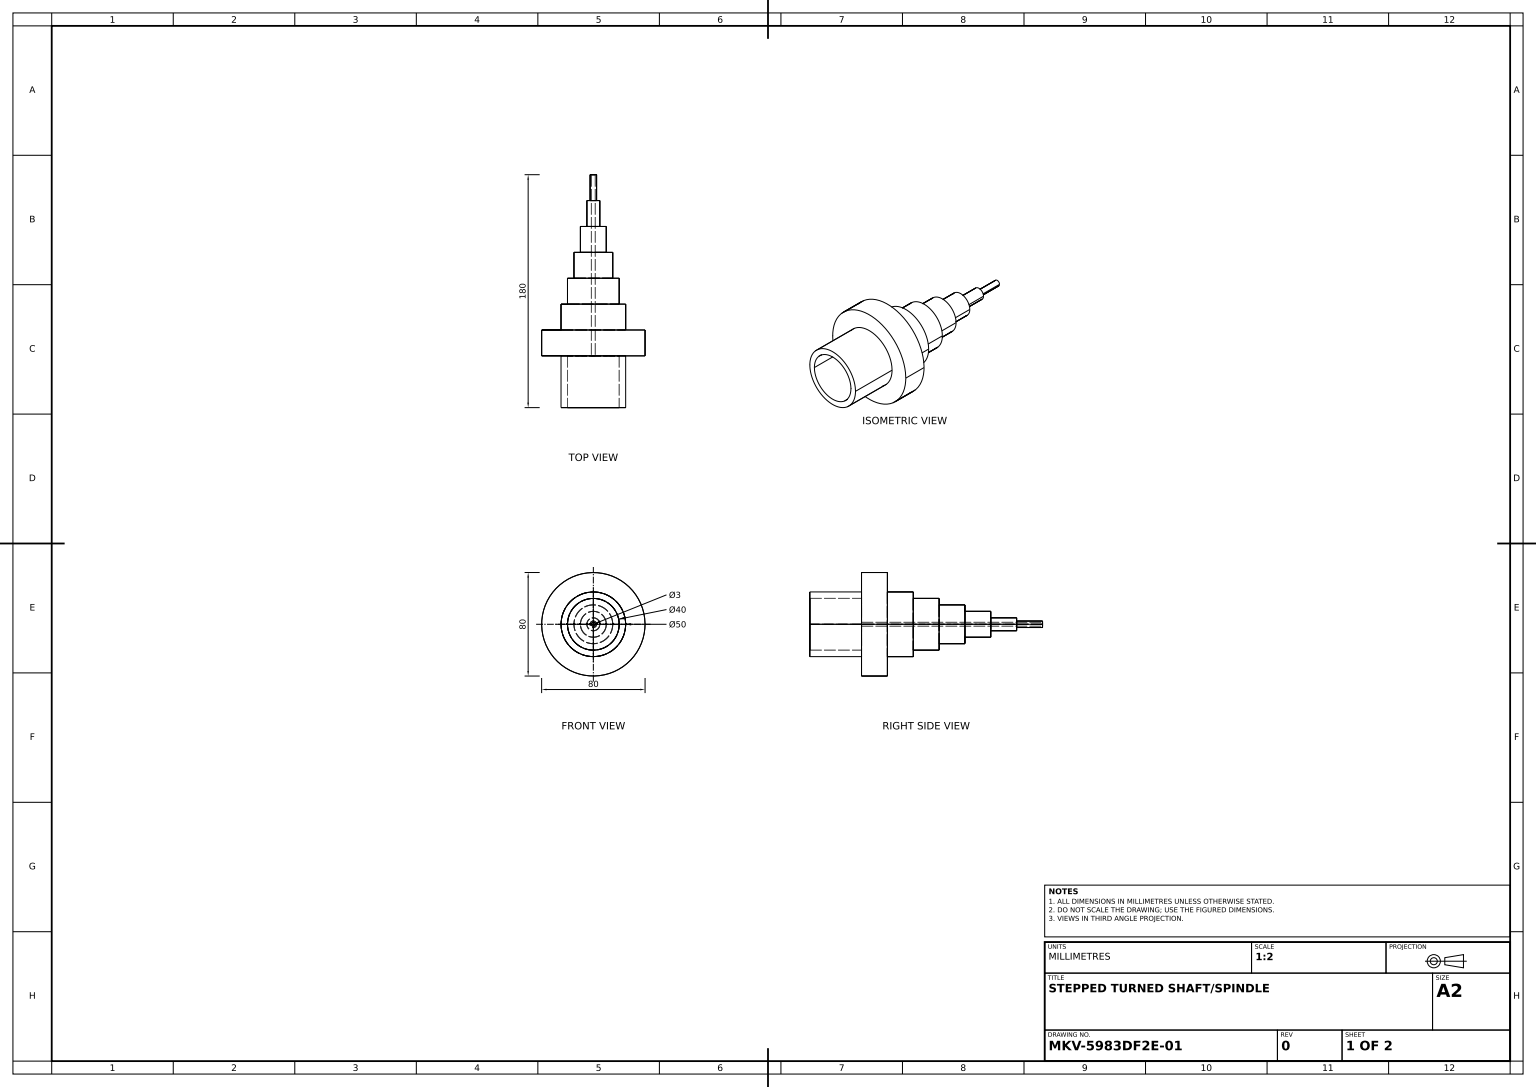
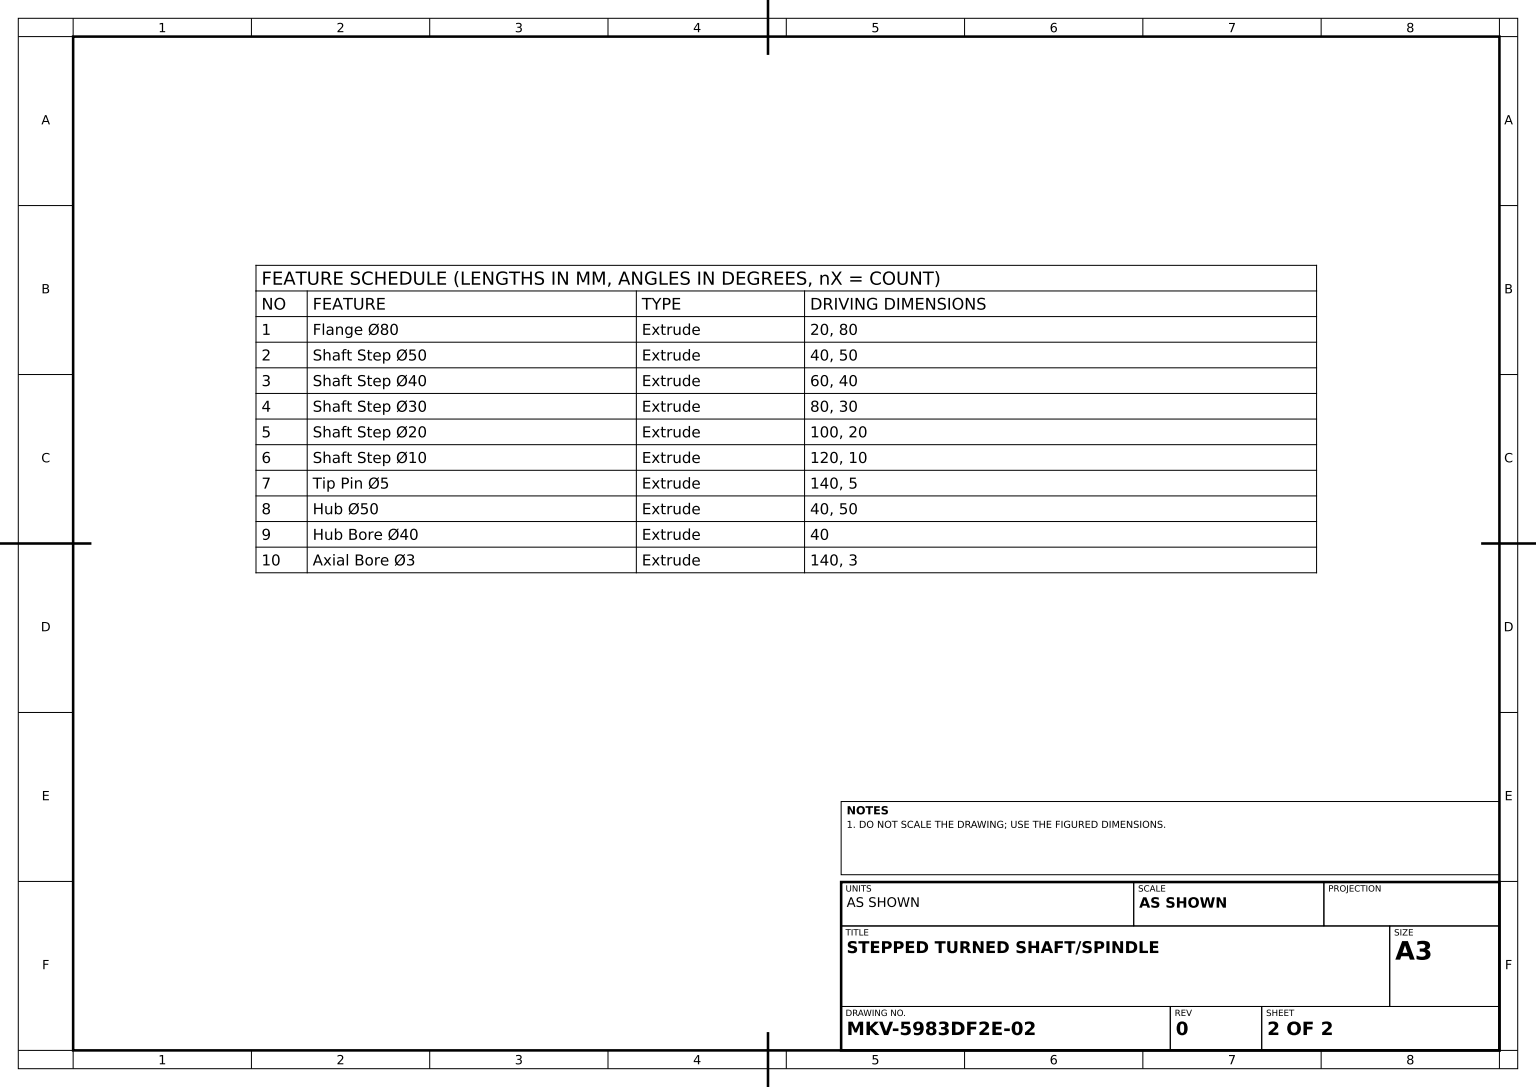
from build123d import *

# Parameters (mm, degrees)
FLANGE_PROFILE_80_R    = 40
FLANGE_80_DEPTH        = 20
STEP_50_PROFILE_R      = 25
SHAFT_STEP_50_DEPTH    = 40
STEP_40_PROFILE_R      = 20
SHAFT_STEP_40_DEPTH    = 60
STEP_30_PROFILE_R      = 15
SHAFT_STEP_30_DEPTH    = 80
STEP_20_PROFILE_R      = 10
SHAFT_STEP_20_DEPTH    = 100
STEP_10_PROFILE_R      = 5
SHAFT_STEP_10_DEPTH    = 120
TIP_PIN_5_PROFILE_R    = 2.5
TIP_PIN_5_DEPTH        = 140
HUB_START              = 40
HUB_50_PROFILE_R       = 25
HUB_50_DEPTH           = 40
HUB_BORE_40_PROFILE_R  = 20
HUB_BORE_40_DEPTH      = 40
AXIAL_BORE_3_PROFILE_R = 1.5
AXIAL_BORE_3_DEPTH     = 140


with BuildPart() as part:
    # Flange Profile Ø80 → Flange Ø80 (new body)
    with BuildSketch(Plane.XY):
        Circle(FLANGE_PROFILE_80_R)
    extrude(amount=-FLANGE_80_DEPTH)

    # Step Ø50 Profile → Shaft Step Ø50 (add)
    with BuildSketch(Plane.XY):
        Circle(STEP_50_PROFILE_R)
    extrude(amount=-SHAFT_STEP_50_DEPTH)

    # Step Ø40 Profile → Shaft Step Ø40 (add)
    with BuildSketch(Plane.XY):
        Circle(STEP_40_PROFILE_R)
    extrude(amount=-SHAFT_STEP_40_DEPTH)

    # Step Ø30 Profile → Shaft Step Ø30 (add)
    with BuildSketch(Plane.XY):
        Circle(STEP_30_PROFILE_R)
    extrude(amount=-SHAFT_STEP_30_DEPTH)

    # Step Ø20 Profile → Shaft Step Ø20 (add)
    with BuildSketch(Plane.XY):
        Circle(STEP_20_PROFILE_R)
    extrude(amount=-SHAFT_STEP_20_DEPTH)

    # Step Ø10 Profile → Shaft Step Ø10 (add)
    with BuildSketch(Plane.XY):
        Circle(STEP_10_PROFILE_R)
    extrude(amount=-SHAFT_STEP_10_DEPTH)

    # Tip Pin Ø5 Profile → Tip Pin Ø5 (add)
    with BuildSketch(Plane.XY):
        Circle(TIP_PIN_5_PROFILE_R)
    extrude(amount=-TIP_PIN_5_DEPTH)

    # Hub Ø50 Profile → Hub Ø50 (add)
    with BuildSketch(Plane.XY.offset(HUB_START)):
        Circle(HUB_50_PROFILE_R)
    extrude(amount=-HUB_50_DEPTH)

    # Hub Bore Ø40 Profile → Hub Bore Ø40 (cut)
    with BuildSketch(Plane.XY.offset(40)):
        Circle(HUB_BORE_40_PROFILE_R)
    extrude(amount=-HUB_BORE_40_DEPTH, mode=Mode.SUBTRACT)

    # Axial Bore Ø3 Profile → Axial Bore Ø3 (cut)
    with BuildSketch(Plane.XY):
        Circle(AXIAL_BORE_3_PROFILE_R)
    extrude(amount=-AXIAL_BORE_3_DEPTH, mode=Mode.SUBTRACT)


solid = part.part
